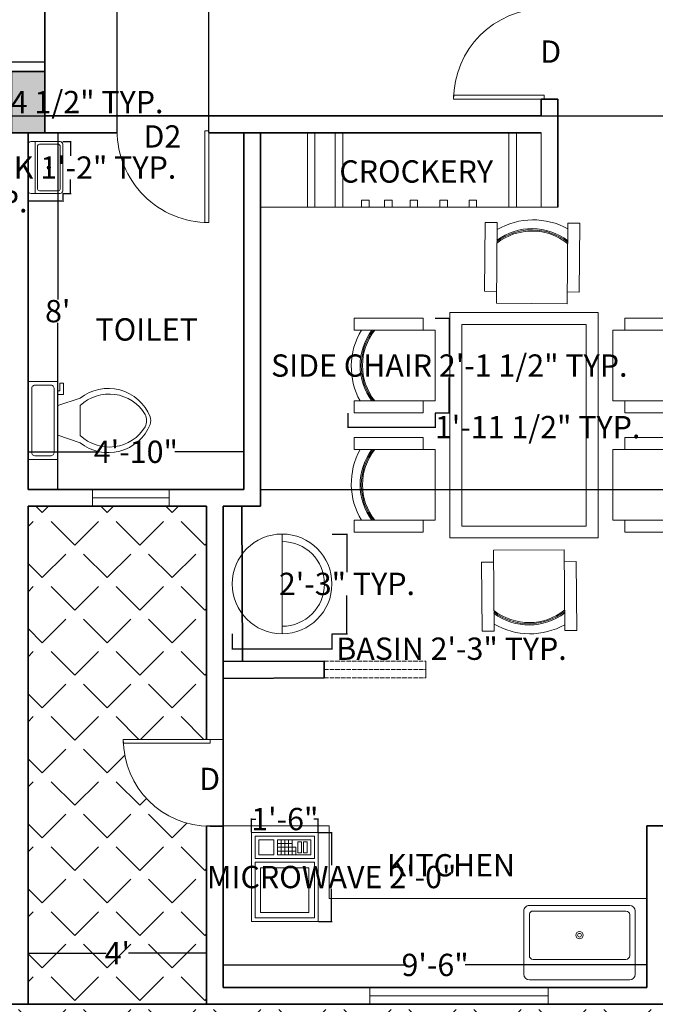
# Model space of a CAD drawing. Units: inches. Extents: x -2181 to 1225, y -80 to 4016.
# Tile 7 of 10: x 668 to 839, y 191 to 456. Entities that reach past the tile are written whole.
import ezdxf

# ---------------------------------------------------------------- set-up
doc = ezdxf.new("R2010")
doc.units = ezdxf.units.IN
doc.header["$MEASUREMENT"] = 0
doc.linetypes.add('ACAD_ISO02W100', pattern=[15, 12, -3])
for name, color, linetype, lineweight in [('A-ANNO-DIMS', 2, 'Continuous', 18), ('A-ANNO-TEXT', 7, 'Continuous', 18), ('A-AREA-IDEN', 7, 'Continuous', 18), ('A-COLS', 7, 'Continuous', 35), ('A-COLS-PATT', 252, 'Continuous', 13), ('A-DOOR', 3, 'Continuous', 18), ('A-EQPM', 9, 'Continuous', 18), ('A-FLOR-FIXT', 8, 'Continuous', 18), ('A-FLOR-PATT', 252, 'Continuous', 13), ('A-FURN', 30, 'Continuous', 18), ('A-GLAZ', 4, 'Continuous', 18), ('A-MILL', 8, 'Continuous', 18), ('A-WALL', 7, 'Continuous', 35), ('A-WALL-OVHD', 7, 'ACAD_ISO02W100', 18)]:
    doc.layers.add(name, color=color, linetype=linetype, lineweight=lineweight)
doc.styles.get("Standard").update_dxf_attribs({"font": 'arial.ttf'})
doc.dimstyles.get("Standard").update_dxf_attribs({"dimtxt": 6, "dimasz": 0.18, "dimexe": 0.18, "dimexo": 0.0625, "dimgap": 0.09, "dimtad": 0, "dimtih": 1, "dimtoh": 1, "dimdec": 4, "dimzin": 0, "dimdsep": 46, "dimlunit": 4, "dimtxsty": 'Standard', "dimcen": 0.09, "dimadec": 0, "dimazin": 0, "dimtfac": 1, "dimtdec": 4, "dimtofl": 0, "dimtmove": 0, "dimatfit": 3, "dimfxl": 1, "dimtolj": 1, "dimtzin": 0, "dimarcsym": 0})
pattern_1 = [(45, (0, 0), (-8.75045, 8.75045), [9, -3.375]), (135, (0, 0), (-8.75045, -8.75045), [9, -3.375])]

# ---------------------------------------------------------------- blocks, each defined once
blk = doc.blocks.new('*U2')
for p, q in [((0, 0), (0, -6)), ((40, 0), (40, -6))]:
    blk.add_line(p, q)
blk.add_lwpolyline([(0, 0), (0, 40), (1.75, 40), (1.75, 0)], close=True)
blk.add_arc((0, 0), 40, 0, 90)
blk = doc.blocks.new('Microwave')
for p, q in [((19, 7), (19, 11)), ((20, 11), (20, 7)), ((21, 7), (21, 11)), ((18, 10), (22, 10)), ((22, 9), (18, 9)), ((18, 8), (22, 8)), ((22, 7), (18, 7)), ((20, 6), (18, 6)), ((19, 6), (19, 7)), ((20, 7), (20, 6))]:
    blk.add_line(p, q)
for points in [[(0, 0), (0, 18), (24, 18), (24, 0)], [(1, 1), (1, 17), (16, 17), (16, 1)], [(17, 1), (17, 17), (23, 17), (23, 1)], [(18, 12), (18, 16), (22, 16), (22, 12)], [(2.5, 2.5), (2.5, 15.5), (14.5, 15.5), (14.5, 2.5)], [(18, 2), (18, 11), (22, 11), (22, 2)], [(18.5, 4.5), (18.5, 5.5), (21.5, 5.5), (21.5, 4.5)], [(18.5, 3), (18.5, 4), (21.5, 4), (21.5, 3)]]:
    blk.add_lwpolyline(points, close=True)
blk = doc.blocks.new('Sink-single - 30 in top')
blk.add_line((-15, -3.999996), (15, -3.999996))
for points in [[(-13.5, 0), (13.5, 0)], [(-15, -18.499996), (-15, -1.5)], [(15, -1.5), (15, -18.499996)], [(-13.5, -17.499996), (-13.5, -6.499996)], [(-12.5, -5.499996), (12.5, -5.499996)], [(13.5, -6.499996), (13.5, -17.499996)], [(12.5, -18.499996), (-12.5, -18.499996)], [(13.5, -19.999996), (-13.5, -19.999996)]]:
    blk.add_lwpolyline(points)
for radius in [1, 0.5]:
    blk.add_circle((0, -11.999996), radius)
for centre, radius, start, end in [((-13.5, -1.5), 1.5, 90, 180), ((13.5, -1.5), 1.5, 0, 90), ((-12.5, -6.499996), 1, 90, 180), ((12.5, -6.499996), 1, 0, 90), ((-13.5, -18.499996), 1.5, 180, 270), ((-12.5, -17.499996), 1, 180, 270), ((12.5, -17.499996), 1, 270, 0), ((13.5, -18.499996), 1.5, 270, 0)]:
    blk.add_arc(centre, radius, start, end)
blk = doc.blocks.new('*U21')
for p, q in [((9.5, -6), (9.5, -2)), ((-10, -8.5), (-8, -8.5)), ((-10, -9.5), (-10, -8.5)), ((-7, -9.5), (-10, -9.5)), ((-8, -8.5), (-8, -8)), ((-7, -8), (-7, -9.5)), ((-4, -8), (-6, -14)), ((4, -8), (6, -14)), ((4, -14), (-4, -14))]:
    blk.add_line(p, q)
blk.add_lwpolyline([(10.5, -8), (10.5, 0), (-10.5, 0), (-10.5, -8)], close=True)
for points in [[(-9.5, -2), (-9.5, -6)], [(8.5, -1), (-8.5, -1)], [(-8.5, -7), (8.5, -7)]]:
    blk.add_lwpolyline(points)
for centre, radius, start, end in [((-8.62, -1.88), 0.884, 81.8699, 188.1301), ((8.62, -1.88), 0.884, 351.8699, 98.1301), ((-8.62, -6.12), 0.884, 171.8699, 278.1301), ((8.62, -6.12), 0.884, 261.8699, 8.1301), ((3.52, -21.58), 12.17, 141.4691, 247.9714), ((4.2, -21.82), 11.33, 136.3677, 238.9468), ((-3.52, -21.58), 12.17, 292.0284, 38.5307), ((-4.2, -21.82), 11.33, 301.053, 43.6321), ((0, -27.88), 4, 245.7318, 294.2682), ((0, -29), 4, 254.8605, 285.1395)]:
    blk.add_arc(centre, radius, start, end)
blk = doc.blocks.new('*D51')
at = {"layer": 'A-ANNO-DIMS', "color": 0, "lineweight": -2, "transparency": 16777216}
for p, q in [((670.08, 425.98), (678.16, 425.98)), ((677.98, 425.8), (677.98, 381.14)), ((677.98, 330.16), (677.98, 374.83)), ((670.08, 329.98), (678.16, 329.98))]:
    blk.add_line(p, q, dxfattribs=at)
at = {"layer": 'A-ANNO-DIMS', "color": 0, "transparency": 16777216}
for points in [[(677.95, 425.8), (678.01, 425.8), (677.98, 425.98)], [(677.95, 330.16), (678.01, 330.16), (677.98, 329.98)]]:
    blk.add_solid(points, dxfattribs=at)
at = {"layer": 'Defpoints', "color": 0, "transparency": 16777216}
for p in [(670.01, 425.98), (670.01, 329.98), (677.98, 329.98)]:
    blk.add_point(p, dxfattribs=at)
at = {"layer": 'A-ANNO-DIMS', "color": 0, "transparency": 16777216, "insert": (677.98, 377.98), "char_height": 6, "attachment_point": 5}
blk.add_mtext("\\A1;8'", dxfattribs=at)
blk = doc.blocks.new('*D52')
at = {"layer": 'A-ANNO-DIMS', "color": 0, "lineweight": -2, "transparency": 16777216}
for p, q in [((670.01, 330.05), (670.01, 340.32)), ((670.19, 340.14), (688.5, 340.14)), ((727.83, 340.14), (709.53, 340.14)), ((728.01, 330.05), (728.01, 340.32))]:
    blk.add_line(p, q, dxfattribs=at)
at = {"layer": 'A-ANNO-DIMS', "color": 0, "transparency": 16777216}
for points in [[(670.19, 340.17), (670.19, 340.11), (670.01, 340.14)], [(727.83, 340.17), (727.83, 340.11), (728.01, 340.14)]]:
    blk.add_solid(points, dxfattribs=at)
at = {"layer": 'Defpoints', "color": 0, "transparency": 16777216}
for p in [(728.01, 340.14), (670.01, 329.98), (728.01, 329.98)]:
    blk.add_point(p, dxfattribs=at)
at = {"layer": 'A-ANNO-DIMS', "color": 0, "transparency": 16777216, "insert": (699.01, 340.14), "char_height": 6, "attachment_point": 5}
blk.add_mtext('\\A1;4\'-10"', dxfattribs=at)
blk = doc.blocks.new('*D56')
at = {"layer": 'A-ANNO-DIMS', "color": 0, "lineweight": -2, "transparency": 16777216}
for p, q in [((722.51, 196.05), (722.51, 202.26)), ((722.69, 202.08), (771.45, 202.08)), ((836.33, 202.08), (787.58, 202.08)), ((836.51, 196.05), (836.51, 202.26))]:
    blk.add_line(p, q, dxfattribs=at)
at = {"layer": 'A-ANNO-DIMS', "color": 0, "transparency": 16777216}
for points in [[(722.69, 202.11), (722.69, 202.05), (722.51, 202.08)], [(836.33, 202.11), (836.33, 202.05), (836.51, 202.08)]]:
    blk.add_solid(points, dxfattribs=at)
at = {"layer": 'Defpoints', "color": 0, "transparency": 16777216}
for p in [(836.51, 202.08), (722.51, 195.98), (836.51, 195.98)]:
    blk.add_point(p, dxfattribs=at)
at = {"layer": 'A-ANNO-DIMS', "color": 0, "transparency": 16777216, "insert": (779.51, 202.08), "char_height": 6, "attachment_point": 5}
blk.add_mtext('\\A1;9\'-6"', dxfattribs=at)
blk = doc.blocks.new('*D57')
at = {"layer": 'A-ANNO-DIMS', "color": 0, "lineweight": -2, "transparency": 16777216}
for p, q in [((732.51, 330.05), (732.51, 330.16)), ((732.69, 329.98), (849.07, 329.98)), ((986.33, 329.98), (869.96, 329.98)), ((986.51, 330.05), (986.51, 330.16))]:
    blk.add_line(p, q, dxfattribs=at)
at = {"layer": 'A-ANNO-DIMS', "color": 0, "transparency": 16777216}
for points in [[(732.69, 330.01), (732.69, 329.95), (732.51, 329.98)], [(986.33, 330.01), (986.33, 329.95), (986.51, 329.98)]]:
    blk.add_solid(points, dxfattribs=at)
at = {"layer": 'Defpoints', "color": 0, "transparency": 16777216}
for p in [(732.51, 329.98), (986.51, 329.98), (986.51, 329.98)]:
    blk.add_point(p, dxfattribs=at)
at = {"layer": 'A-ANNO-DIMS', "color": 0, "transparency": 16777216, "insert": (859.51, 329.98), "char_height": 6, "attachment_point": 5}
blk.add_mtext('\\A1;21\'-2"', dxfattribs=at)
blk = doc.blocks.new('*D62')
at = {"layer": 'A-ANNO-DIMS', "color": 0, "lineweight": -2, "transparency": 16777216}
for p, q in [((670.01, 191.55), (670.01, 205.4)), ((670.19, 205.22), (691.04, 205.22)), ((717.83, 205.22), (696.99, 205.22)), ((718.01, 191.55), (718.01, 205.4))]:
    blk.add_line(p, q, dxfattribs=at)
at = {"layer": 'A-ANNO-DIMS', "color": 0, "transparency": 16777216}
for points in [[(670.19, 205.25), (670.19, 205.19), (670.01, 205.22)], [(717.83, 205.25), (717.83, 205.19), (718.01, 205.22)]]:
    blk.add_solid(points, dxfattribs=at)
at = {"layer": 'Defpoints', "color": 0, "transparency": 16777216}
for p in [(718.01, 205.22), (670.01, 191.48), (718.01, 191.48)]:
    blk.add_point(p, dxfattribs=at)
at = {"layer": 'A-ANNO-DIMS', "color": 0, "transparency": 16777216, "insert": (694.01, 205.22), "char_height": 6, "attachment_point": 5}
blk.add_mtext("\\A1;4'", dxfattribs=at)
blk = doc.blocks.new('DINING-CHAIR-SIDE')
for p, q in [((0.79, 22.26), (0.79, 25.47)), ((19.33, 22.26), (19.33, 25.47)), ((0.79, 0), (0.79, 3.21)), ((19.33, 3.21), (19.33, 0))]:
    blk.add_line(p, q)
for points in [[(0.79, 25.47), (19.33, 25.47)], [(0.79, 22.26), (22.53, 22.26), (22.53, 3.21), (0.79, 3.21)], [(19.33, 0), (0.79, 0)]]:
    blk.add_lwpolyline(points)
for centre, radius, start, end in [((19.12, 12.45), 19.13, 149.1418, 208.8973), ((18.29, 12.73), 15.92, 143.2428, 216.7572), ((18.29, 12.73), 15.6, 142.3578, 217.6422), ((18.29, 12.73), 15.28, 141.4242, 218.5758)]:
    blk.add_arc(centre, radius, start, end)
blk = doc.blocks.new('DINING-CHAIR-END')
for p, q in [((3.21, 19.25), (0, 19.23)), ((22.26, 19.4), (25.47, 19.42)), ((25.38, 19.42), (25.38, 19.34)), ((3.35, 0.72), (0.14, 0.69)), ((25.61, 0.89), (22.4, 0.86))]:
    blk.add_line(p, q)
for points in [[(3.35, 0.72), (3.18, 22.46), (22.23, 22.61), (22.4, 0.86)], [(0.14, 0.69), (0, 19.23)], [(25.47, 19.42), (25.61, 0.89)]]:
    blk.add_lwpolyline(points)
for centre, radius, start, end in [((12.74, 18.29), 15.28, 231.8612, 309.0129), ((12.74, 18.29), 15.6, 232.7948, 308.0793), ((12.74, 18.29), 15.92, 233.6799, 307.1942), ((13.02, 19.13), 19.13, 239.5789, 299.3344)]:
    blk.add_arc(centre, radius, start, end)
blk = doc.blocks.new('DINING-TABLE')
for points in [[(39.83, 60.67), (39.83, 0), (0, 0), (0, 60.67)], [(36.62, 57.46), (36.62, 3.21), (3.21, 3.21), (3.21, 57.46)]]:
    blk.add_lwpolyline(points, close=True)
blk = doc.blocks.new('BASIN-ROUND')
blk.add_line((13.41, 0), (13.41, 26.83))
blk.add_circle((13.41, 13.41), 13.41)
blk.add_arc((13.41, 13.41), 11.41, 270, 90)
blk = doc.blocks.new('COL-16.5X9')
blk.add_lwpolyline([(0, 16.5), (9, 16.5), (9, 0), (0, 0)], close=True)
blk = doc.blocks.new('*D92')
at = {"layer": 'A-ANNO-DIMS', "color": 0, "lineweight": -2, "transparency": 16777216}
for p, q in [((679.38, 423.59), (681.59, 423.59)), ((681.41, 423.41), (681.41, 419.8)), ((681.41, 409.82), (681.41, 413.42)), ((679.38, 409.64), (681.59, 409.64))]:
    blk.add_line(p, q, dxfattribs=at)
at = {"layer": 'A-ANNO-DIMS', "color": 0, "transparency": 16777216}
for points in [[(681.38, 423.41), (681.44, 423.41), (681.41, 423.59)], [(681.38, 409.82), (681.44, 409.82), (681.41, 409.64)]]:
    blk.add_solid(points, dxfattribs=at)
at = {"layer": 'Defpoints', "color": 0, "transparency": 16777216}
for p in [(679.31, 423.59), (679.31, 409.64), (681.41, 409.64)]:
    blk.add_point(p, dxfattribs=at)
at = {"layer": 'A-ANNO-DIMS', "color": 0, "transparency": 16777216, "insert": (681.41, 416.61), "char_height": 6, "attachment_point": 5}
blk.add_mtext('\\A1;SINK 1\'-2" TYP.', dxfattribs=at)
blk = doc.blocks.new('*D93')
at = {"layer": 'A-ANNO-DIMS', "color": 0, "lineweight": -2, "transparency": 16777216}
for p, q in [((670.01, 409.57), (670.01, 407.36)), ((679.31, 409.57), (679.31, 407.36)), ((670.01, 407.54), (669.83, 407.54)), ((679.13, 407.54), (670.19, 407.54))]:
    blk.add_line(p, q, dxfattribs=at)
at = {"layer": 'A-ANNO-DIMS', "color": 0, "transparency": 16777216}
for points in [[(670.19, 407.57), (670.19, 407.51), (670.01, 407.54)], [(679.13, 407.57), (679.13, 407.51), (679.31, 407.54)]]:
    blk.add_solid(points, dxfattribs=at)
at = {"layer": 'Defpoints', "color": 0, "transparency": 16777216}
for p in [(670.01, 409.64), (679.31, 409.64), (670.01, 407.54)]:
    blk.add_point(p, dxfattribs=at)
at = {"layer": 'A-ANNO-DIMS', "color": 0, "transparency": 16777216, "insert": (644.47, 407.54), "char_height": 6, "attachment_point": 5}
blk.add_mtext('\\A1;0\'-9 1/2" TYP.', dxfattribs=at)
blk = doc.blocks.new('*D94')
at = {"layer": 'A-ANNO-DIMS', "color": 0, "lineweight": -2, "transparency": 16777216}
for p, q in [((779.57, 376.07), (783.51, 376.07)), ((783.33, 375.89), (783.33, 366.53)), ((783.33, 350.78), (783.33, 360.15)), ((779.57, 350.6), (783.51, 350.6))]:
    blk.add_line(p, q, dxfattribs=at)
at = {"layer": 'A-ANNO-DIMS', "color": 0, "transparency": 16777216}
for points in [[(783.3, 375.89), (783.36, 375.89), (783.33, 376.07)], [(783.3, 350.78), (783.36, 350.78), (783.33, 350.6)]]:
    blk.add_solid(points, dxfattribs=at)
at = {"layer": 'Defpoints', "color": 0, "transparency": 16777216}
for p in [(779.51, 376.07), (783.33, 376.07), (779.51, 350.6)]:
    blk.add_point(p, dxfattribs=at)
at = {"layer": 'A-ANNO-DIMS', "color": 0, "transparency": 16777216, "insert": (783.33, 363.34), "char_height": 6, "attachment_point": 5}
blk.add_mtext('\\A1;SIDE CHAIR 2\'-1 1/2" TYP.', dxfattribs=at)
blk = doc.blocks.new('*D95')
at = {"layer": 'A-ANNO-DIMS', "color": 0, "lineweight": -2, "transparency": 16777216}
for p, q in [((756.06, 350.54), (756.06, 346.6)), ((779.51, 350.54), (779.51, 346.6)), ((756.24, 346.78), (779.33, 346.78)), ((779.51, 346.78), (779.69, 346.78))]:
    blk.add_line(p, q, dxfattribs=at)
at = {"layer": 'A-ANNO-DIMS', "color": 0, "transparency": 16777216}
for points in [[(756.24, 346.81), (756.24, 346.75), (756.06, 346.78)], [(779.33, 346.81), (779.33, 346.75), (779.51, 346.78)]]:
    blk.add_solid(points, dxfattribs=at)
at = {"layer": 'Defpoints', "color": 0, "transparency": 16777216}
for p in [(756.06, 350.6), (779.51, 350.6), (779.51, 346.78)]:
    blk.add_point(p, dxfattribs=at)
at = {"layer": 'A-ANNO-DIMS', "color": 0, "transparency": 16777216, "insert": (807.1, 346.78), "char_height": 6, "attachment_point": 5}
blk.add_mtext('\\A1;1\'-11 1/2" TYP.', dxfattribs=at)
blk = doc.blocks.new('*D104')
at = {"layer": 'A-ANNO-DIMS', "color": 0, "lineweight": -2, "transparency": 16777216}
for p, q in [((665.45, 442.48), (662.86, 442.48)), ((663.04, 442.3), (663.04, 437.43)), ((663.04, 426.16), (663.04, 431.04)), ((665.45, 425.98), (662.86, 425.98))]:
    blk.add_line(p, q, dxfattribs=at)
at = {"layer": 'A-ANNO-DIMS', "color": 0, "transparency": 16777216}
for points in [[(663.01, 442.3), (663.07, 442.3), (663.04, 442.48)], [(663.01, 426.16), (663.07, 426.16), (663.04, 425.98)]]:
    blk.add_solid(points, dxfattribs=at)
at = {"layer": 'Defpoints', "color": 0, "transparency": 16777216}
for p in [(665.51, 442.48), (663.04, 425.98), (665.51, 425.98)]:
    blk.add_point(p, dxfattribs=at)
at = {"layer": 'A-ANNO-DIMS', "color": 0, "transparency": 16777216, "insert": (663.04, 434.23), "char_height": 6, "attachment_point": 5}
blk.add_mtext('\\A1;COLUMN 1\'-4 1/2" TYP.', dxfattribs=at)
blk = doc.blocks.new('*D105')
at = {"layer": 'A-ANNO-DIMS', "color": 0, "lineweight": -2, "transparency": 16777216}
for p, q in [((665.51, 442.55), (665.51, 445.14)), ((674.51, 442.55), (674.51, 445.14)), ((665.51, 444.96), (665.33, 444.96)), ((674.33, 444.96), (665.69, 444.96))]:
    blk.add_line(p, q, dxfattribs=at)
at = {"layer": 'A-ANNO-DIMS', "color": 0, "transparency": 16777216}
for points in [[(665.69, 444.99), (665.69, 444.93), (665.51, 444.96)], [(674.33, 444.99), (674.33, 444.93), (674.51, 444.96)]]:
    blk.add_solid(points, dxfattribs=at)
at = {"layer": 'Defpoints', "color": 0, "transparency": 16777216}
for p in [(665.51, 444.96), (665.51, 442.48), (674.51, 442.48)]:
    blk.add_point(p, dxfattribs=at)
at = {"layer": 'A-ANNO-DIMS', "color": 0, "transparency": 16777216, "insert": (646.96, 444.96), "char_height": 6, "attachment_point": 5}
blk.add_mtext('\\A1;0\'-9" TYP.', dxfattribs=at)
blk = doc.blocks.new('*D112')
at = {"layer": 'A-ANNO-DIMS', "color": 0, "lineweight": -2, "transparency": 16777216}
for p, q in [((724.93, 291.12), (724.93, 286.98)), ((751.76, 291.12), (751.76, 286.98)), ((725.11, 287.16), (751.58, 287.16)), ((751.76, 287.16), (751.94, 287.16))]:
    blk.add_line(p, q, dxfattribs=at)
at = {"layer": 'A-ANNO-DIMS', "color": 0, "transparency": 16777216}
for points in [[(725.11, 287.19), (725.11, 287.13), (724.93, 287.16)], [(751.58, 287.19), (751.58, 287.13), (751.76, 287.16)]]:
    blk.add_solid(points, dxfattribs=at)
at = {"layer": 'Defpoints', "color": 0, "transparency": 16777216}
for p in [(724.93, 291.18), (751.76, 291.18), (751.76, 287.16)]:
    blk.add_point(p, dxfattribs=at)
at = {"layer": 'A-ANNO-DIMS', "color": 0, "transparency": 16777216, "insert": (783.93, 287.16), "char_height": 6, "attachment_point": 5}
blk.add_mtext('\\A1;BASIN 2\'-3" TYP.', dxfattribs=at)
blk = doc.blocks.new('*D113')
at = {"layer": 'A-ANNO-DIMS', "color": 0, "lineweight": -2, "transparency": 16777216}
for p, q in [((751.83, 318.01), (755.97, 318.01)), ((755.79, 317.83), (755.79, 307.75)), ((755.79, 291.36), (755.79, 301.44)), ((751.83, 291.18), (755.97, 291.18))]:
    blk.add_line(p, q, dxfattribs=at)
at = {"layer": 'A-ANNO-DIMS', "color": 0, "transparency": 16777216}
for points in [[(755.76, 317.83), (755.82, 317.83), (755.79, 318.01)], [(755.76, 291.36), (755.82, 291.36), (755.79, 291.18)]]:
    blk.add_solid(points, dxfattribs=at)
at = {"layer": 'Defpoints', "color": 0, "transparency": 16777216}
for p in [(751.76, 318.01), (755.79, 318.01), (751.76, 291.18)]:
    blk.add_point(p, dxfattribs=at)
at = {"layer": 'A-ANNO-DIMS', "color": 0, "transparency": 16777216, "insert": (755.79, 304.6), "char_height": 6, "attachment_point": 5}
blk.add_mtext('\\A1;2\'-3" TYP.', dxfattribs=at)
blk = doc.blocks.new('*D128')
at = {"layer": 'A-ANNO-DIMS', "color": 0, "lineweight": -2, "transparency": 16777216}
for p, q in [((748.14, 237.73), (751.86, 237.73)), ((751.68, 237.55), (751.68, 228.92)), ((751.68, 213.91), (751.68, 222.53)), ((748.14, 213.73), (751.86, 213.73))]:
    blk.add_line(p, q, dxfattribs=at)
at = {"layer": 'A-ANNO-DIMS', "color": 0, "transparency": 16777216}
for points in [[(751.65, 237.55), (751.71, 237.55), (751.68, 237.73)], [(751.65, 213.91), (751.71, 213.91), (751.68, 213.73)]]:
    blk.add_solid(points, dxfattribs=at)
at = {"layer": 'Defpoints', "color": 0, "transparency": 16777216}
for p in [(748.08, 237.73), (751.68, 237.73), (748.08, 213.73)]:
    blk.add_point(p, dxfattribs=at)
at = {"layer": 'A-ANNO-DIMS', "color": 0, "transparency": 16777216, "insert": (751.68, 225.73), "char_height": 6, "attachment_point": 5}
blk.add_mtext('\\A1;MICROWAVE 2\'-0"', dxfattribs=at)
blk = doc.blocks.new('*D129')
at = {"layer": 'A-ANNO-DIMS', "color": 0, "lineweight": -2, "transparency": 16777216}
for p, q in [((730.08, 237.79), (730.08, 241.51)), ((730.26, 241.33), (731.3, 241.33)), ((747.9, 241.33), (746.86, 241.33)), ((748.08, 237.79), (748.08, 241.51))]:
    blk.add_line(p, q, dxfattribs=at)
at = {"layer": 'A-ANNO-DIMS', "color": 0, "transparency": 16777216}
for points in [[(730.26, 241.36), (730.26, 241.3), (730.08, 241.33)], [(747.9, 241.36), (747.9, 241.3), (748.08, 241.33)]]:
    blk.add_solid(points, dxfattribs=at)
at = {"layer": 'Defpoints', "color": 0, "transparency": 16777216}
for p in [(730.08, 241.33), (730.08, 237.73), (748.08, 237.73)]:
    blk.add_point(p, dxfattribs=at)
at = {"layer": 'A-ANNO-DIMS', "color": 0, "transparency": 16777216, "insert": (739.08, 241.33), "char_height": 6, "attachment_point": 5}
blk.add_mtext('\\A1;1\'-6"', dxfattribs=at)
blk = doc.blocks.new('*D131')
at = {"layer": 'A-ANNO-DIMS', "color": 0, "lineweight": -2, "transparency": 16777216}
for p, q in [((976.64, 563.98), (-59.44, 563.98)), ((-59.26, 563.8), (-59.26, 500.43)), ((-59.26, 430.66), (-59.26, 494.04)), ((977.45, 430.48), (-59.44, 430.48))]:
    blk.add_line(p, q, dxfattribs=at)
at = {"layer": 'A-ANNO-DIMS', "color": 0, "transparency": 16777216}
for points in [[(-59.29, 563.8), (-59.23, 563.8), (-59.26, 563.98)], [(-59.29, 430.66), (-59.23, 430.66), (-59.26, 430.48)]]:
    blk.add_solid(points, dxfattribs=at)
at = {"layer": 'Defpoints', "color": 0, "transparency": 16777216}
for p in [(976.7, 563.98), (-59.26, 430.48), (977.51, 430.48)]:
    blk.add_point(p, dxfattribs=at)
at = {"layer": 'A-ANNO-DIMS', "color": 0, "transparency": 16777216, "insert": (-59.26, 497.23), "char_height": 6, "attachment_point": 5}
blk.add_mtext('\\A1;11\'-1 1/2"', dxfattribs=at)
blk = doc.blocks.new('*D134')
at = {"layer": 'A-ANNO-DIMS', "color": 0, "lineweight": -2, "transparency": 16777216}
for p, q in [((693.95, 426.05), (693.95, 726.81)), ((694.13, 726.63), (718.45, 726.63)), ((718.63, 426.05), (718.63, 726.81)), ((718.63, 726.63), (718.81, 726.63))]:
    blk.add_line(p, q, dxfattribs=at)
at = {"layer": 'A-ANNO-DIMS', "color": 0, "transparency": 16777216}
for points in [[(694.13, 726.66), (694.13, 726.6), (693.95, 726.63)], [(718.45, 726.66), (718.45, 726.6), (718.63, 726.63)]]:
    blk.add_solid(points, dxfattribs=at)
at = {"layer": 'Defpoints', "color": 0, "transparency": 16777216}
for p in [(718.63, 726.63), (693.95, 425.98), (718.63, 425.98)]:
    blk.add_point(p, dxfattribs=at)
at = {"layer": 'A-ANNO-DIMS', "color": 0, "transparency": 16777216, "insert": (733.91, 726.63), "char_height": 6, "attachment_point": 5}
blk.add_mtext('\\A1;2\'-0 1/2"', dxfattribs=at)

msp = doc.modelspace()

# ---------------------------------------------------------------- hatches: boundary and pattern name
at = {"layer": 'A-COLS-PATT'}
h = msp.add_hatch(color=256, dxfattribs=at)
h.dxf.hatch_style = 1
h.paths.add_polyline_path([(995.51461, 209.98479), (986.51461, 209.98479), (986.51461, 191.48479), (995.51461, 191.48479)])
h.paths.add_polyline_path([(862.50488, 191.48479), (862.50488, 200.48479), (841.01461, 200.48479), (841.01461, 191.48479)])
h.paths.add_polyline_path([(995.51461, 425.98479), (995.51461, 434.98479), (977.51461, 434.98479), (977.51461, 425.98479)])
h.paths.add_polyline_path([(880.01461, 425.98479), (880.01461, 432.54138), (862.01461, 432.54138), (862.01461, 425.98479)])
h.paths.add_polyline_path([(880.82546, 563.98479), (880.82546, 572.98479), (862.01461, 572.98479), (862.01461, 563.98479)])
h.paths.add_polyline_path([(995.51461, 563.98479), (995.51461, 572.98479), (976.70377, 572.98479), (976.70377, 563.98479)])
h.paths.add_polyline_path([(674.51461, 572.98479), (665.51461, 572.98479), (665.51461, 556.48479), (674.51461, 556.48479)])
h.paths.add_polyline_path([(674.51461, 442.48479), (665.51461, 442.48479), (665.51461, 425.98479), (674.51461, 425.98479)])
at = {"layer": 'A-FLOR-PATT'}
h = msp.add_hatch(dxfattribs=at)
h.set_pattern_fill('ANGLE', color=256, scale=45, angle=45)
h.set_pattern_definition(pattern_1)
h.paths.add_polyline_path([(718.01461, 239.37925, -0.389216795), (695.62809, 261.73364), (695.60569, 261.73364), (695.60569, 262.75735), (718.01461, 262.75735), (718.01461, 325.48479), (670.01461, 325.48479), (670.01461, 191.48479), (718.01461, 191.48479)])
h = msp.add_hatch(dxfattribs=at)
h.set_pattern_fill('ANGLE', color=256, scale=45, angle=45)
h.set_pattern_definition(pattern_1)
h.paths.add_polyline_path([(665.51461, 191.48479), (665.51461, 136.48479), (674.51461, 136.48479), (674.51461, 137.48479), (994.51461, 137.48479), (994.51461, 191.48479)])

# ---------------------------------------------------------------- linework, layer by layer
at = {"layer": 'A-GLAZ'}
for p, q in [((687.36479, 329.98479), (687.36479, 325.48479)), ((707.98713, 329.98479), (707.98713, 325.48479)), ((687.36479, 327.73479), (707.98713, 327.73479)), ((761.96891, 195.98479), (761.96891, 191.48479)), ((761.96891, 193.73479), (809.96891, 193.73479)), ((809.96891, 195.98479), (809.96891, 191.48479))]:
    msp.add_line(p, q, dxfattribs=at)
at = {"layer": 'A-MILL'}
for p, q in [((745.14164, 425.98479), (745.14164, 405.98479)), ((747.14164, 425.98479), (747.14164, 405.98479)), ((752.66987, 405.98479), (752.66987, 425.98479)), ((754.66987, 405.98479), (754.66987, 425.98479)), ((799.39907, 405.98479), (799.39907, 425.98479)), ((801.39907, 405.98479), (801.39907, 425.98479)), ((759.75526, 405.98479), (759.75526, 407.84973)), ((759.75526, 407.84973), (761.75526, 407.84973)), ((761.75526, 405.98479), (761.75526, 407.84973)), ((765.94131, 405.98479), (765.94131, 407.84973)), ((765.94131, 407.84973), (767.94131, 407.84973)), ((767.94131, 405.98479), (767.94131, 407.84973)), ((772.76461, 405.98479), (772.76461, 407.84973)), ((772.76461, 407.84973), (774.76461, 407.84973)), ((774.76461, 405.98479), (774.76461, 407.84973)), ((780.81784, 405.98479), (780.81784, 407.84973)), ((780.81784, 407.84973), (782.81784, 407.84973)), ((782.81784, 405.98479), (782.81784, 407.84973)), ((788.64715, 405.98479), (788.64715, 407.84973)), ((788.64715, 407.84973), (790.64715, 407.84973)), ((790.64715, 405.98479), (790.64715, 407.84973)), ((718.01461, 239.47545), (751.0146, 239.50967)), ((751.0146, 239.50967), (751.0146, 219.98479))]:
    msp.add_line(p, q, dxfattribs=at)
for points in [[(808.01461, 405.98479), (808.01461, 425.98479)], [(732.51461, 405.98479), (812.51461, 405.98479)], [(751.0146, 219.98479), (836.51461, 219.98479)]]:
    msp.add_lwpolyline(points, dxfattribs=at)
at = {"layer": 'A-WALL'}
for p, q in [((732.51461, 329.98479), (732.51461, 325.48479)), ((727.51461, 325.48479), (727.70693, 283.70956)), ((722.51461, 294.41862), (722.51461, 300.85056)), ((722.4939, 283.68556), (749.64933, 283.81058)), ((749.67005, 279.31062), (749.64933, 283.81058)), ((722.51461, 279.18561), (749.67005, 279.31062)), ((836.51461, 239.48479), (841.01461, 239.48479))]:
    msp.add_line(p, q, dxfattribs=at)
for points in [[(674.51461, 425.98479), (674.51461, 563.98479)], [(812.51461, 434.98479), (808.01461, 434.98479)], [(808.01461, 430.48479), (808.01461, 434.98479)], [(812.51461, 405.98479), (812.51461, 434.98479)], [(808.01461, 430.48479), (674.51461, 430.48479)], [(701.17814, 430.48479), (674.51461, 430.48479)], [(808.01461, 430.48479), (737.01461, 430.48479)], [(693.94574, 425.98479), (665.51461, 425.98479)], [(670.01461, 329.98479), (670.01461, 425.98479)], [(732.51461, 425.98479), (718.62705, 425.98479)], [(728.01461, 329.98479), (728.01461, 425.98479)], [(732.51461, 329.98479), (732.51461, 425.98479)], [(808.01461, 425.98479), (732.51461, 425.98479)], [(728.01461, 329.98479), (670.01461, 329.98479)], [(670.01461, 191.48479), (670.01461, 325.48479)], [(718.01461, 325.48479), (670.01461, 325.48479)], [(718.01461, 262.75735), (718.01461, 325.48479)], [(732.51461, 325.48479), (722.51461, 325.48479)], [(722.51461, 283.68566), (722.51461, 325.48479)], [(722.51461, 195.98479), (722.51461, 300.85056)], [(722.51461, 262.75735), (722.51461, 279.18561)], [(718.01461, 191.48479), (718.01461, 239.47545)], [(836.51461, 195.98479), (836.51461, 239.48479)], [(722.51461, 195.98479), (836.51461, 195.98479)], [(665.51461, 191.48479), (995.51461, 191.48479)]]:
    msp.add_lwpolyline(points, dxfattribs=at)
at = {"layer": 'A-WALL-OVHD', "ltscale": 0.1}
for p, q in [((749.64933, 283.81058), (777.04315, 283.81058)), ((749.65969, 281.5606), (777.04315, 281.5606)), ((749.67005, 279.31062), (777.04315, 279.31062))]:
    msp.add_line(p, q, dxfattribs=at)
at = {"layer": 'A-WALL-OVHD'}
msp.add_line((777.04315, 283.81058), (777.04315, 279.31062), dxfattribs=at)

# ---------------------------------------------------------------- block references
at = {"layer": 'A-COLS', "rotation": 180}
msp.add_blockref('COL-16.5X9', (674.51423, 442.48457), dxfattribs=at)
at = {"layer": 'A-DOOR'}
for p, xscale, yscale, zscale, rotation in [((808.86196, 434.98479), 0.608774911433326, 0.608774911433326, 0.608774911433326, 90.00000000000003), ((718.6267, 426.52675), 0.617172616085525, 0.617172616085525, 0.617172616085525, 180.0380366063734)]:
    msp.add_blockref('*U2', p, dxfattribs=dict(at, xscale=xscale, yscale=yscale, zscale=zscale, rotation=rotation))
at = {"layer": 'A-DOOR', "extrusion": (0, 0, -1), "xscale": 0.5849766441292635, "yscale": 0.5849766441292635, "zscale": -0.5849766441292635, "rotation": 270}
msp.add_blockref('*U2', (-719.00475, 262.75735), dxfattribs=at)
at = {"layer": 'A-EQPM', "rotation": 90}
msp.add_blockref('Microwave', (748.08147, 213.72664), dxfattribs=at)
at = {"layer": 'A-FLOR-FIXT', "xscale": -0.4649637902209482, "yscale": 0.4649637902209482, "zscale": 0.4649637902209482, "rotation": 90}
msp.add_blockref('Sink-single - 30 in top', (670.01461, 416.61086), dxfattribs=at)
at = {"layer": 'A-FLOR-FIXT', "xscale": -1, "rotation": 89.90827745497215}
msp.add_blockref('*U21', (669.99609, 348.58544), dxfattribs=at)
at = {"layer": 'A-FLOR-FIXT'}
msp.add_blockref('BASIN-ROUND', (724.934, 291.183), dxfattribs=at)
at = {"layer": 'A-FLOR-FIXT', "rotation": 180}
msp.add_blockref('Sink-single - 30 in top', (818.37233, 198.07696), dxfattribs=at)
at = {"layer": 'A-FURN', "extrusion": (0, 0, -1), "zscale": -1, "rotation": 180}
for name, p in [('DINING-CHAIR-END', (-792.84967, 402.54373)), ('DINING-CHAIR-SIDE', (-756.971, 343.96907))]:
    msp.add_blockref(name, p, dxfattribs=at)
at = {"layer": 'A-FURN'}
for name, p in [('DINING-TABLE', (783.522, 316.953)), ('DINING-CHAIR-SIDE', (756.971, 350.605)), ('DINING-CHAIR-END', (792.0332, 291.17077))]:
    msp.add_blockref(name, p, dxfattribs=at)
at = {"layer": 'A-FURN', "extrusion": (0, 0, -1), "zscale": -1}
msp.add_blockref('DINING-CHAIR-SIDE', (-849.90472, 350.605), dxfattribs=at)
at = {"layer": 'A-FURN', "rotation": 180}
msp.add_blockref('DINING-CHAIR-SIDE', (849.90472, 343.96907), dxfattribs=at)

# ---------------------------------------------------------------- texts
at = {"layer": 'A-ANNO-TEXT', "char_height": 6, "attachment_point": 1}
for s, insert in [('D', (807.80081, 450.81476)), ('D2', (701.05479, 427.98122)), ('CROCKERY', (753.74644, 418.55418)), ('D', (716.0311, 255.12811))]:
    msp.add_mtext_dynamic_manual_height_columns(s, width=291.4178321, gutter_width=1, heights=[0], dxfattribs=dict(at, insert=insert))
at = {"layer": 'A-AREA-IDEN', "char_height": 6, "attachment_point": 1}
for s, insert in [('TOILET', (688.13615, 376.05281)), ('KITCHEN', (766.51484, 231.89089))]:
    msp.add_mtext_dynamic_manual_height_columns(s, width=291.4178321, gutter_width=1, heights=[0], dxfattribs=dict(at, insert=insert))

# ---------------------------------------------------------------- dimensions: what is measured, and where the dimension line sits
at = {"layer": 'A-ANNO-DIMS'}
for base, p1, p2, override, picture, middle in [((718.62706, 726.63478), (693.94574, 425.98478), (718.62706, 425.98478), {"dimdec": 1, "dimlfac": 1, "dimrnd": 0, "dimzin": 1, "dimdsep": 46, "dimlunit": 4, "dimfrac": 2}, '*D134', (733.91343, 726.63478)), ((728.01461, 340.13558), (670.01461, 329.98479), (728.01461, 329.98479), {"dimclrd": 0, "dimclre": 0, "dimclrt": 0}, '*D52', (699.01461, 340.13558)), ((986.51461, 329.98479), (732.51461, 329.98479), (986.51461, 329.98479), {"dimclrd": 0, "dimclre": 0, "dimclrt": 0}, '*D57', (859.51461, 329.98479)), ((718.01461, 205.22043), (670.01461, 191.48479), (718.01461, 191.48479), {"dimclrd": 0, "dimclre": 0, "dimclrt": 0}, '*D62', (694.01461, 205.22043)), ((836.51461, 202.07695), (722.51461, 195.98479), (836.51461, 195.98479), {"dimclrd": 0, "dimclre": 0, "dimclrt": 0}, '*D56', (779.51461, 202.07695))]:
    dim = msp.add_linear_dim(base=base, p1=p1, p2=p2, dimstyle='Standard', override=override, dxfattribs=at)
    dim.commit()
    dim.dimension.update_dxf_attribs({"geometry": picture, "text_midpoint": middle})
for base, p1, p2, angle, override, picture, middle in [((-59.2566, 430.48478), (976.70377, 563.98478), (977.51461, 430.48478), 90, {"dimdec": 1, "dimlfac": 1, "dimrnd": 0, "dimzin": 1, "dimdsep": 46, "dimlunit": 4, "dimfrac": 2}, '*D131', (-59.2566, 497.23478)), ((677.97927, 329.98479), (670.01461, 425.98479), (670.01461, 329.98479), 90, {"dimclrd": 0, "dimclre": 0, "dimclrt": 0}, '*D51', (677.97927, 377.98479)), ((730.08147, 241.32664), (748.08147, 237.72664), (730.08147, 237.72664), 180, {"dimdec": 1, "dimlfac": 1, "dimrnd": 0, "dimzin": 1, "dimdsep": 46, "dimlunit": 4, "dimfrac": 2}, '*D129', (739.08147, 241.32664))]:
    dim = msp.add_linear_dim(base=base, p1=p1, p2=p2, angle=angle, dimstyle='Standard', override=override, dxfattribs=at)
    dim.commit()
    dim.dimension.update_dxf_attribs({"geometry": picture, "text_midpoint": middle})
for base, p1, p2, angle, text, picture, middle in [((663.03961, 425.98479), (665.51461, 442.48479), (665.51461, 425.98479), 270, 'COLUMN <> TYP.', '*D104', (663.03961, 434.23479)), ((665.51461, 444.95979), (674.51461, 442.48479), (665.51461, 442.48479), 180, '<> TYP.', '*D105', (646.95812, 444.95979)), ((681.40622, 409.6364), (679.31389, 423.58532), (679.31389, 409.6364), 270, 'SINK <> TYP.', '*D92', (681.40622, 416.61086)), ((670.01461, 407.54407), (679.31389, 409.6364), (670.01461, 409.6364), 180, '<> TYP.', '*D93', (644.46767, 407.54407)), ((783.32547, 376.07208), (779.50534, 350.60458), (779.50534, 376.07208), 90, 'SIDE CHAIR <> TYP.', '*D94', (783.32547, 363.33833)), ((755.78722, 318.01142), (751.76295, 291.18292), (751.76295, 318.01142), 90, '<> TYP.', '*D113', (755.78722, 304.59717)), ((751.68147, 237.72664), (748.08147, 213.72664), (748.08147, 237.72664), 90, 'MICROWAVE <>', '*D128', (751.68147, 225.72664))]:
    dim = msp.add_linear_dim(base=base, p1=p1, p2=p2, angle=angle, text=text, dimstyle='Standard', override={"dimdec": 1, "dimlfac": 1, "dimrnd": 0, "dimzin": 1, "dimdsep": 46, "dimlunit": 4, "dimfrac": 2}, dxfattribs=at)
    dim.commit()
    dim.dimension.update_dxf_attribs({"geometry": picture, "text_midpoint": middle})
for base, p1, p2, text, picture, middle in [((779.50534, 346.78446), (756.0618, 350.60458), (779.50534, 350.60458), '<> TYP.', '*D95', (807.10072, 346.78446)), ((751.76295, 287.15865), (724.93445, 291.18292), (751.76295, 291.18292), 'BASIN <> TYP.', '*D112', (783.9279, 287.15865))]:
    dim = msp.add_linear_dim(base=base, p1=p1, p2=p2, text=text, dimstyle='Standard', override={"dimdec": 1, "dimlfac": 1, "dimrnd": 0, "dimzin": 1, "dimdsep": 46, "dimlunit": 4, "dimfrac": 2}, dxfattribs=at)
    dim.commit()
    dim.dimension.update_dxf_attribs({"geometry": picture, "text_midpoint": middle})

doc.saveas('drawing.dxf')
